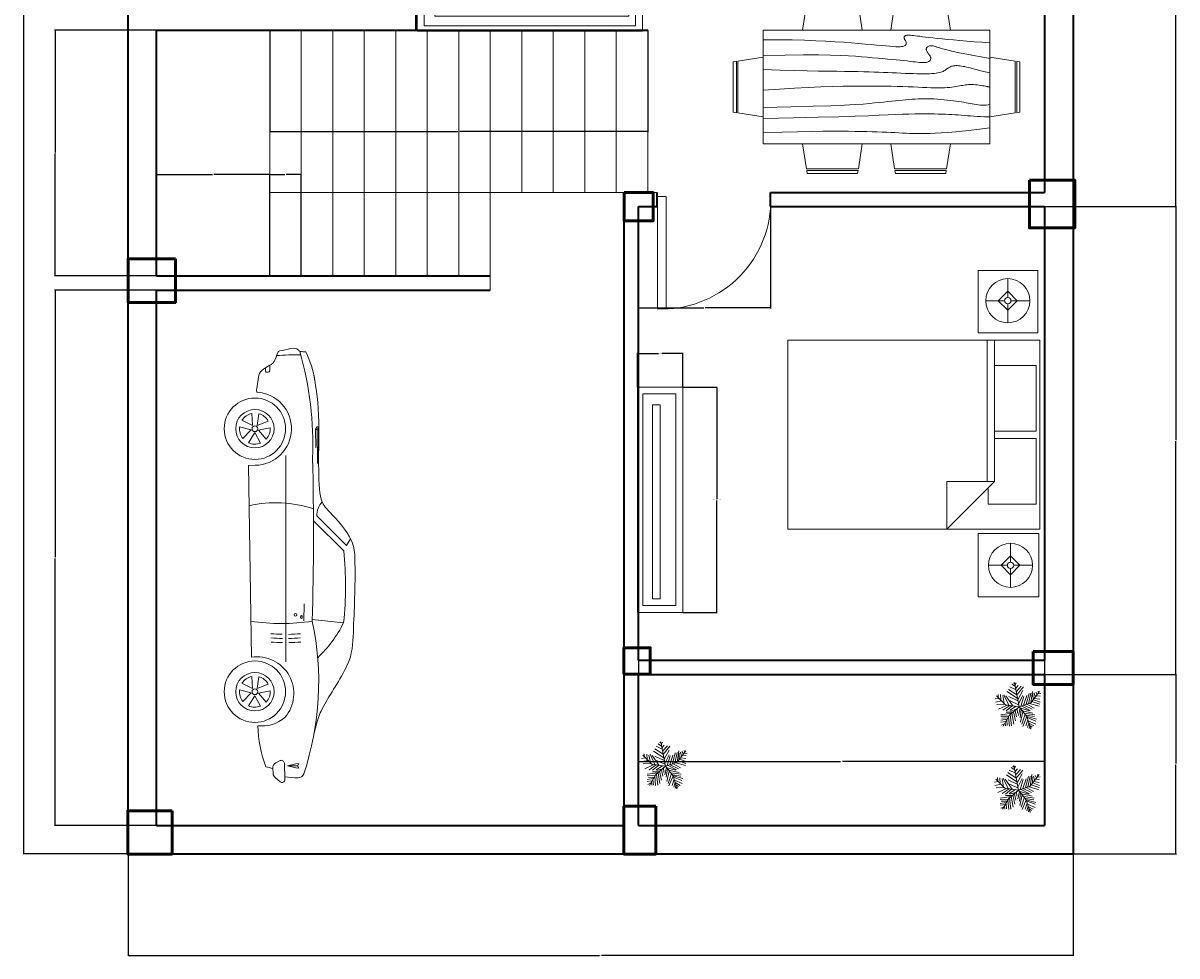
# Model space of a CAD drawing. Units: inches. Extents: x 50 to 2003, y -28 to 675.
# Tile 1 of 10: x 179 to 545, y -15 to 281. Entities that reach past the tile are written whole.
import ezdxf

# ---------------------------------------------------------------- set-up
doc = ezdxf.new("R2010")
doc.units = ezdxf.units.IN
for name, color, linetype, lineweight in [('A-ANNO-DIMS', 2, 'Continuous', 18), ('A-COLS', 1, 'Continuous', 50), ('A-DOOR', 4, 'Continuous', 18), ('A-FLOR-STRS', 4, 'Continuous', 18), ('A-FURN', 8, 'Continuous', 18), ('A-FURN-LITE', 9, 'Continuous', 13), ('A-SITE-VEHC', 8, 'Continuous', 13), ('A-WALL', 7, 'Continuous', 35), ('L-PLNT', 3, 'Continuous', 13)]:
    doc.layers.add(name, color=color, linetype=linetype, lineweight=lineweight)
doc.styles.get("Standard").update_dxf_attribs({"font": 'arial.ttf'})
doc.dimstyles.get("Standard").update_dxf_attribs({"dimtxt": 0.18, "dimasz": 0.18, "dimexe": 0.18, "dimexo": 0.0625, "dimgap": 0.09, "dimtad": 0, "dimtih": 1, "dimtoh": 1, "dimdec": 4, "dimzin": 0, "dimdsep": 46, "dimtxsty": 'Standard', "dimcen": 0.09, "dimadec": 0, "dimazin": 0, "dimtfac": 1, "dimtdec": 4, "dimtofl": 0, "dimtmove": 0, "dimatfit": 3, "dimfxl": 1, "dimtolj": 1, "dimtzin": 0, "dimarcsym": 0})

# ---------------------------------------------------------------- blocks, each defined once
blk = doc.blocks.new('*U4')
for p, q in [((72.93, 40.23), (85.8, 53.18)), ((75, 38.82), (88.08, 51.97)), ((119.39, 51.91), (117.92, 38.32)), ((50.13, 41.06), (34.31, 40.98)), ((35.3, 40.46), (50.13, 40.62)), ((43.26, 39.85), (35.15, 39.78)), ((111.09, 34.73), (118.48, 34.64)), ((46.65, 26.83), (136.29, 26.77)), ((180.37, 26.17), (187.51, 26.41)), ((179.3, 24.35), (180.25, 22.49)), ((182.62, 21.14), (184.91, 21.28)), ((186.68, 22.17), (188.51, 24.37)), ((7.45, 19.78), (9.74, 19.8)), ((9.76, 17.93), (8.53, 17.92)), ((10.37, 19.19), (10.38, 18.56)), ((50.87, 13.52), (50.91, 10.52))]:
    blk.add_line(p, q)
for points in [[(35.31, 39.93), (35.3, 40.27, 0.269532), (35.14, 40.54), (34.38, 40.96, 0.575383), (34.15, 40.83), (34.15, 40.49, 0.269532), (34.32, 40.22), (35.08, 39.79, 0.575383)], [(28.49, 15.1), (33.61, 14.4), (31.65, 19.18, 0.199906)], [(34.64, 20.05), (35.56, 14.97), (39.5, 18.31, 0.199906)], [(41.25, 15.74), (36.7, 13.3), (41.09, 10.58, 0.199906)], [(142.85, 15.1), (147.96, 14.4), (146.01, 19.18, 0.199906)], [(148.99, 20.05), (149.91, 14.97), (153.85, 18.31, 0.199906)], [(155.6, 15.74), (151.06, 13.3), (155.45, 10.58, 0.199906)], [(31.31, 7.72), (33.55, 12.37), (28.4, 11.99, 0.199906)], [(39.19, 8.12), (35.46, 11.69), (34.23, 6.67, 0.199906)], [(145.66, 7.72), (147.9, 12.37), (142.75, 11.99, 0.199906)], [(153.54, 8.12), (149.81, 11.69), (148.59, 6.67, 0.199906)]]:
    blk.add_lwpolyline(points, format="xyb", close=True)
for points in [[(181.58, 27.46), (181.53, 31.95), (180.48, 32.43)], [(181.58, 27.46), (181.53, 31.95), (182.57, 32.45)], [(50.91, 10.52), (134.38, 11.83)]]:
    blk.add_lwpolyline(points)
for centre, radius in [((115.89, 31.01), 0.619), ((34.98, 13.35), 13.35), ((149.33, 13.35), 13.35), ((34.98, 13.35), 8.35), ((149.33, 13.35), 8.35), ((34.98, 13.35), 1.25), ((149.33, 13.35), 1.25)]:
    blk.add_circle(centre, radius)
for centre, radius, start, end in [((114.6, 105.09), 59.37, 237.6103, 240.9785), ((103.45, -95), 147.78, 83.8163, 95.9705), ((95.51, 3.91), 53.61, 43.2748, 63.5665), ((73.29, 50.49), 10.26, 230.424, 268.0085), ((145.17, -84.88), 125.99, 71.5283, 102.1242), ((42.18, -111.35), 149.91, 87.8393, 105.8096), ((20.53, -3.15), 43.06, 98.5304, 116.112), ((80.1, -1364.13), 1402.96, 88.42296, 91.3179), ((118.31, 22.51), 51.16, 161.4307, 193.2363), ((25.66, 24.94), 94.01, 351.8279, 8.1674), ((79.16, 30.11), 76.3, 177.5773, 185.5205), ((45.64, 26.83), 78.76, 0.852, 4.6556), ((47.43, 26.85), 78.76, 0.852, 4.6556), ((49.23, 26.87), 78.76, 0.852, 4.6556), ((150.1, 14.36), 15.92, 49.2263, 189.1528), ((216.26, 37.76), 36.17, 188.4683, 196.5315), ((146.68, 36.98), 36.17, 344.7432, 352.8063), ((184.3, 32.25), 2.49, 357.932, 71.5283), ((116.55, 34.7), 70.29, 353.1942, 357.932), ((34.98, 13.35), 15.9, 0.6373, 176.3412), ((45.64, 26.83), 78.76, 355.2644, 358.8633), ((47.43, 26.85), 78.76, 355.2644, 358.8633), ((49.23, 26.87), 78.76, 355.2644, 358.8633), ((149.4, 16.55), 14.84, 352.7285, 41.6613), ((180.41, 24.92), 1.25, 91.939, 207.109), ((187.55, 25.16), 1.25, 320.1683, 91.939), ((182.47, 23.63), 2.49, 207.109, 273.4677), ((114.25, 37.03), 70.29, 344.3985, 346.9385), ((184.76, 23.76), 2.49, 273.4677, 320.1683), ((9.75, 19.18), 0.623, 0.6373, 90.6373), ((9.76, 18.55), 0.623, 270.6373, 0.6373), ((162.47, 70.82), 56.18, 271.6865, 290.2774)]:
    blk.add_arc(centre, radius, start, end)
blk.add_ellipse((116.89, 33.59), major_axis=(-0.63, -0.007), ratio=0.610043)
for points, knots in [([(11.39, 38.92), (18.06, 40.19), (30.91, 42.01), (64.77, 40.11), (70.25, 44.91), (82.35, 56.38), (99.18, 57.3), (116.06, 56.35), (133.04, 55.87), (145.24, 49.87), (153.62, 43.8), (161.17, 40.68), (164.92, 39.73), (167.29, 39.15)], [18.629823, 18.629823, 18.629823, 18.629823, 19.527405, 20.700571, 21.107983, 21.608568, 21.92336, 23.151359, 23.716171, 23.908743, 24.77794, 24.943072, 25.187755, 25.187755, 25.187755, 25.187755]), ([(19.11, 14.36), (18.99, 14.21), (18.5, 13.81), (15.35, 15), (9.19, 13.94), (7.26, 22.22), (3.01, 22.66), (1.32, 23.61), (0.64, 26.92), (-0.96, 31.49), (1.54, 32.64), (1.5, 34.06), (1.49, 34.8), (1.49, 35.06), (1.52, 35.3), (1.58, 35.51)], [16.815853, 16.815853, 16.815853, 16.815853, 16.838212, 16.885395, 17.18439, 17.479846, 17.654423, 17.670693, 17.696923, 18.016358, 18.052739, 18.140805, 18.140805, 18.140805, 18.172382, 18.172382, 18.172382, 18.172382])]:
    blk.add_open_spline(points, degree=3, knots=knots)
blk = doc.blocks.new('*U2')
for p, q in [((-10.186, 53.64), (-13.084, 55.962)), ((0, 0), (-10.5, 57)), ((-9.099, 51.782), (-6.563, 55.962)), ((-48.585, 21.131), (-49.309, 29.026)), ((-43.513, 28.561), (-42.427, 15.558)), ((-35.544, 28.097), (-24.314, 3.947)), ((-3.665, 19.273), (-27.574, 35.527)), ((-5.114, 28.097), (-24.676, 40.636)), ((-7.288, 39.707), (-21.778, 46.673)), ((-8.737, 47.138), (-17.069, 52.711)), ((-7.65, 43.423), (-2.578, 49.46)), ((-5.839, 35.992), (4.667, 48.067)), ((-5.114, 27.632), (10.463, 46.673)), ((-2.941, 16.486), (8.652, 37.85)), ((16.259, 5.805), (23.142, 31.348)), ((22.055, 7.198), (27.489, 32.277)), ((27, 9), (48, 36)), ((27.127, 9.056), (31.112, 35.992)), ((31.836, 30.883), (32.561, 16.486)), ((35.096, 32.741), (37.27, 22.524)), ((38.719, 34.134), (41.979, 28.561)), ((43.791, 29.954), (51.036, 30.883)), ((44.153, 36.456), (45.239, 32.741)), ((-47.498, 19.737), (-55.83, 18.344)), ((-40.615, 13.7), (-55.105, 10.913)), ((-31.5, 4.5), (-52.5, 25.5)), ((-33.37, 6.269), (-52.207, 5.34)), ((-28.299, 3.483), (-47.86, -5.805)), ((-38.442, 26.239), (-34.819, 7.663)), ((-21.416, 3.018), (-38.079, -8.128)), ((0, 0), (-31.5, 4.5)), ((-14.533, 2.09), (-30.834, 25.31)), ((-15.982, 2.09), (-30.11, -9.521)), ((-24.314, 23.917), (-2.941, 13.7)), ((0, 0), (-22.5, -19.5)), ((-6.563, 1.161), (-21.416, -8.128)), ((-20.691, 13.7), (-1.129, 4.876)), ((-1.129, 6.734), (9.014, 26.704)), ((0, 0), (27, 9)), ((0, 0), (18, -22.5)), ((3.942, 1.625), (11.187, 24.381)), ((6.478, 1.625), (26.04, -8.592)), ((10.101, 3.483), (17.708, 26.239)), ((11.187, 3.483), (30.749, -5.805)), ((18.07, 5.805), (35.096, -3.483)), ((24.229, 7.663), (46.688, 1.625)), ((29.662, 12.307), (48.137, 6.269)), ((33.285, 16.486), (48.862, 10.913)), ((36.183, 19.737), (48.137, 17.88)), ((40.53, 25.775), (48.862, 24.846)), ((-17.431, -15.094), (-42.789, -18.809)), ((-24.314, -21.596), (-42.427, -22.06)), ((-26.849, -26.24), (-40.253, -25.775)), ((-22.5, -19.5), (-37.5, -45)), ((-15.257, -12.772), (-30.11, -12.772)), ((-25.038, -23.918), (-22.865, -45.281)), ((-20.691, -18.345), (-17.793, -44.352)), ((-6.563, -5.805), (-19.967, -9.985)), ((-17.069, -15.094), (-12.721, -40.172)), ((-13.446, -11.378), (-8.737, -32.741)), ((-9.461, -8.592), (-6.201, -23.453)), ((-4.752, -3.483), (-3.665, -14.629)), ((2.493, -3.019), (-1.491, -20.202)), ((1.769, -2.555), (24.229, -9.521)), ((5.029, -6.27), (2.131, -25.775)), ((9.014, -11.378), (3.58, -35.992)), ((14.085, -16.951), (6.478, -40.172)), ((7.565, -9.056), (32.198, -14.629)), ((18.07, -22.524), (8.289, -45.745)), ((12.274, -15.094), (36.907, -18.809)), ((16.259, -19.738), (36.183, -22.989)), ((18, -22.5), (27, -52.5)), ((18.433, -22.524), (40.53, -29.026)), ((19.157, -25.311), (38.719, -33.206)), ((-28.299, -29.026), (-42.789, -31.348)), ((-30.834, -34.135), (-42.427, -35.528)), ((-34.457, -39.708), (-40.978, -42.494)), ((-32.646, -36.921), (-31.921, -44.352)), ((-29.023, -30.884), (-27.936, -43.887)), ((20.244, -30.419), (15.897, -44.816)), ((22.78, -37.85), (19.519, -48.532)), ((21.331, -32.741), (39.081, -40.636)), ((22.78, -38.314), (34.372, -44.816)), ((24.591, -45.745), (23.142, -50.854)), ((24.591, -43.423), (30.749, -47.603)), ((26.764, -49.925), (28.213, -50.854))]:
    blk.add_line(p, q)
blk = doc.blocks.new('Bed - Queen')
for p, q in [((0, -80.00003), (0, 0)), ((0, 0), (59.99999, 0)), ((59.99999, 0), (59.99999, -80.00003)), ((7.99999, -1.2), (28.79998, -1.2)), ((7.99999, -14.4), (7.99999, -1.2)), ((28.79998, -1.2), (28.79998, -14.4)), ((31.19999, -1.2), (51.99999, -1.2)), ((31.19999, -14.4), (31.19999, -1.2)), ((51.99999, -1.2), (51.99999, -16.4)), ((0, -14.4), (44.8, -14.4)), ((59.99999, -29.6), (44.8, -14.4)), ((44.8, -14.4), (44.8, -29.6)), ((44.8, -16.8), (0, -16.8)), ((51.99999, -16.4), (46.79936, -16.4)), ((44.8, -29.6), (59.99999, -29.6)), ((59.99999, -80.00003), (0, -80.00003))]:
    blk.add_line(p, q)
blk = doc.blocks.new('Lamp - Table')
for p, q in [((0, 7), (0, 1)), ((-1, 0), (-7, 0)), ((0, 3), (-3, 0)), ((-3, 0), (0, -3)), ((3, 0), (0, 3)), ((0, -3), (3, 0)), ((1, 0), (7, 0)), ((0, -1), (0, -7))]:
    blk.add_line(p, q)
for radius in [7, 1]:
    blk.add_circle((0, 0), radius)
blk = doc.blocks.new('Dining Set - 36 x 72 in.')
for p, q in [((-22.2343, 26.00059), (-23.4847, 17.99762)), ((-22.2304, 26), (-5.7608, 26)), ((-22, 27.5), (-22.1562, 26.50042)), ((-5.8416, 26.5), (-22.1534, 26.5)), ((-22, 27.5), (-6, 27.5)), ((-5.8437, 26.49966), (-6, 27.5)), ((-4.5152, 17.99762), (-5.7655, 25.99926)), ((5.7657, 26.00059), (4.5153, 17.99762)), ((5.7696, 26), (22.2392, 26)), ((6, 27.5), (5.8438, 26.50042)), ((22.1584, 26.5), (5.8466, 26.5)), ((6, 27.5), (22, 27.5)), ((22.1563, 26.49966), (22, 27.5)), ((23.4848, 17.99762), (22.2345, 25.99926)), ((36, 18), (-36, 18)), ((-36, 18), (-36, -18)), ((36, -18), (36, 18)), ((-45.5, 8), (-44.5004, 8.15617)), ((-45.5, 8), (-45.5, -8)), ((-44.5, -8.15843), (-44.5, 8.15338)), ((-44.0006, 8.23428), (-35.9976, 9.48474)), ((-44, 8.23041), (-44, -8.23915)), ((44.0006, 8.23428), (35.9976, 9.48474)), ((44, 8.23041), (44, -8.23915)), ((44.5, -8.15843), (44.5, 8.15338)), ((45.5, 8), (44.5005, 8.15617)), ((45.5, 8), (45.5, -8)), ((-44.4997, -8.15631), (-45.5, -8)), ((-35.9976, -9.48476), (-43.9993, -8.2345)), ((35.9976, -9.48476), (43.9993, -8.2345)), ((44.4997, -8.15631), (45.5, -8)), ((-36, -18), (36, -18)), ((-22.2343, -26.0006), (-23.4847, -17.99762)), ((-4.5152, -17.99762), (-5.7655, -25.99928)), ((5.7657, -26.0006), (4.5153, -17.99762)), ((23.4848, -17.99762), (22.2345, -25.99928)), ((-22.2304, -26), (-5.7608, -26)), ((-22, -27.5), (-22.1562, -26.50044)), ((-5.8416, -26.5), (-22.1534, -26.5)), ((-22, -27.5), (-6, -27.5)), ((-5.8437, -26.49967), (-6, -27.5)), ((5.7696, -26), (22.2392, -26)), ((6, -27.5), (5.8438, -26.50044)), ((22.1584, -26.5), (5.8466, -26.5)), ((6, -27.5), (22, -27.5)), ((22.1563, -26.49967), (22, -27.5))]:
    blk.add_line(p, q)
for points in [[(-36, 15), (-31.1772, 14.97754), (-26.8079, 14.91406), (-22.8538, 14.81543), (-19.276, 14.6875), (-16.0362, 14.53613), (-13.0957, 14.36718), (-10.4159, 14.18652), (-7.9583, 14), (-5.6904, 13.81315), (-3.6035, 13.63021), (-1.6954, 13.45508), (0.0365, 13.29166), (1.5945, 13.14388), (2.9811, 13.01562), (4.1988, 12.9108), (5.25, 12.83333), (6.1393, 12.78613), (6.8802, 12.76823), (7.4883, 12.77767), (7.9792, 12.8125), (8.3685, 12.87077), (8.6719, 12.95052), (8.9049, 13.0498), (9.0833, 13.16666), (9.2205, 13.29899), (9.3216, 13.44401), (9.3895, 13.59879), (9.4271, 13.76041), (9.4373, 13.92594), (9.4232, 14.09245), (9.3875, 14.257), (9.3333, 14.41666), (9.2638, 14.56917), (9.1836, 14.71484), (9.0975, 14.85465), (9.0104, 14.98958), (8.9272, 15.1206), (8.8529, 15.2487), (8.7922, 15.37483), (8.75, 15.5), (8.7305, 15.62467), (8.7344, 15.74739), (8.7617, 15.86621), (8.8125, 15.97916), (8.8867, 16.08431), (8.9844, 16.17968), (9.1055, 16.26334), (9.25, 16.33333), (9.4189, 16.38802), (9.6172, 16.42708), (9.8506, 16.45052), (10.125, 16.45833), (10.4463, 16.45052), (10.8203, 16.42708), (11.2529, 16.38802), (11.75, 16.33333), (12.3184, 16.26318), (12.9694, 16.17838), (13.7151, 16.07991), (14.5677, 15.96875), (15.5395, 15.84586), (16.6426, 15.71224), (17.8893, 15.56884), (19.2917, 15.41666), (20.859, 15.25667), (22.5879, 15.08984), (24.4721, 14.91715), (26.5052, 14.73958), (28.6809, 14.5581), (30.9929, 14.3737), (33.4347, 14.18733), (36, 14)], [(-36, 10), (-28.9766, 10.14274), (-23.1725, 10.20442), (-18.4241, 10.19775), (-14.5677, 10.13541), (-11.4399, 10.03011), (-8.877, 9.89453), (-6.7154, 9.74137), (-4.7917, 9.58333), (-2.9698, 9.43082), (-1.2246, 9.28515), (0.4415, 9.14534), (2.026, 9.01041), (3.5266, 8.87939), (4.9408, 8.7513), (6.266, 8.62516), (7.5, 8.5), (8.6411, 8.37549), (9.6914, 8.2539), (10.6538, 8.13818), (11.5312, 8.03125), (12.3267, 7.93603), (13.043, 7.85547), (13.6831, 7.79248), (14.25, 7.75), (14.7471, 7.7303), (15.1797, 7.73307), (15.5537, 7.75732), (15.875, 7.80208), (16.1494, 7.86637), (16.3828, 7.94922), (16.5811, 8.04964), (16.75, 8.16666), (16.8944, 8.29915), (17.0143, 8.44531), (17.1089, 8.60319), (17.1771, 8.77083), (17.218, 8.94629), (17.2305, 9.1276), (17.2137, 9.31282), (17.1667, 9.5), (17.0895, 9.6875), (16.987, 9.875), (16.8649, 10.0625), (16.7292, 10.25), (16.5856, 10.4375), (16.4401, 10.625), (16.2985, 10.8125), (16.1667, 11), (16.05, 11.18733), (15.9518, 11.3737), (15.8752, 11.5581), (15.8229, 11.73958), (15.798, 11.91715), (15.8034, 12.08984), (15.842, 12.25667), (15.9167, 12.41666), (16.0295, 12.56836), (16.1784, 12.70833), (16.3605, 12.83268), (16.5729, 12.9375), (16.8127, 13.01888), (17.0768, 13.07291), (17.3625, 13.0957), (17.6667, 13.08333), (17.9894, 13.03312), (18.3418, 12.94726), (18.7382, 12.82918), (19.1927, 12.68229), (19.7195, 12.51001), (20.3327, 12.31575), (21.0465, 12.10294), (21.875, 11.875), (22.8357, 11.63354), (23.959, 11.37304), (25.2786, 11.08618), (26.8282, 10.76562), (28.6414, 10.40405), (30.752, 9.99414), (33.1936, 9.52856), (36, 9)], [(-36, 5.5), (-30.7157, 5.3348), (-26.069, 5.20963), (-21.9946, 5.11767), (-18.4271, 5.05208), (-15.3009, 5.00602), (-12.5508, 4.97265), (-10.1112, 4.94515), (-7.9167, 4.91666), (-5.909, 4.88167), (-4.0586, 4.83984), (-2.3429, 4.79215), (-0.7396, 4.73958), (0.7739, 4.6831), (2.22, 4.6237), (3.6213, 4.56233), (5, 4.5), (6.373, 4.43782), (7.7344, 4.3776), (9.0723, 4.32129), (10.375, 4.27083), (11.6309, 4.22819), (12.8281, 4.19531), (13.9551, 4.17415), (15, 4.16666), (15.954, 4.17448), (16.819, 4.19791), (17.6001, 4.23698), (18.3021, 4.29166), (18.9299, 4.36198), (19.4883, 4.44791), (19.9823, 4.54948), (20.4167, 4.66666), (20.7969, 4.79899), (21.1302, 4.94401), (21.4245, 5.09879), (21.6875, 5.26041), (21.9271, 5.42594), (22.1511, 5.59245), (22.3672, 5.757), (22.5834, 5.91666), (22.8065, 6.06868), (23.0404, 6.21093), (23.2879, 6.34147), (23.5521, 6.45833), (23.8358, 6.55957), (24.142, 6.64323), (24.4735, 6.70735), (24.8334, 6.75), (25.2235, 6.76969), (25.642, 6.76692), (26.0858, 6.74267), (26.5521, 6.69791), (27.0379, 6.63362), (27.5404, 6.55078), (28.0565, 6.45036), (28.5834, 6.33333), (29.1242, 6.19987), (29.7071, 6.04687), (30.3661, 5.87044), (31.1354, 5.66666), (32.0493, 5.43164), (33.142, 5.16146), (34.4475, 4.85221), (36, 4.5)], [(-36, -1), (-30.7915, -0.6591), (-26.0195, -0.38216), (-21.6519, -0.16284), (-17.6563, 0.00521), (-14.0005, 0.12833), (-10.6523, 0.21289), (-7.5796, 0.26522), (-4.75, 0.29166), (-2.134, 0.29793), (0.2878, 0.28711), (2.5317, 0.26163), (4.6146, 0.22396), (6.5529, 0.17651), (8.3633, 0.12174), (10.0623, 0.06209), (11.6667, 0), (13.1899, -0.06201), (14.6341, -0.1211), (15.9982, -0.17432), (17.2813, -0.21875), (18.4823, -0.25147), (19.6003, -0.26953), (20.6343, -0.27002), (21.5834, -0.25), (22.4481, -0.20768), (23.2357, -0.14584), (23.9549, -0.06836), (24.6146, 0.02083), (25.2235, 0.11784), (25.7904, 0.21875), (26.3241, 0.31966), (26.8334, 0.41666), (27.3265, 0.50618), (27.8099, 0.58593), (28.2894, 0.65397), (28.7709, 0.70833), (29.2601, 0.74707), (29.763, 0.76823), (30.2855, 0.76985), (30.8334, 0.75), (31.4088, 0.70784), (31.9994, 0.64713), (32.589, 0.57275), (33.1615, 0.48958), (33.7008, 0.4025), (34.1908, 0.3164), (34.6153, 0.23616), (34.9584, 0.16666), (35.2099, 0.11165), (35.3848, 0.07031), (35.504, 0.04069), (35.5886, 0.02083), (35.6594, 0.00879), (35.7377, 0.0026), (35.8442, 0.00032), (36, 0)], [(-36, -6.5), (-27.1843, -6.31267), (-20.084, -6.1263), (-14.469, -5.9419), (-10.1094, -5.76042), (-6.7752, -5.58285), (-4.2363, -5.41016), (-2.2629, -5.24333), (-0.625, -5.08334), (0.8708, -4.93099), (2.2715, -4.78646), (3.5872, -4.64974), (4.8281, -4.52084), (6.0046, -4.39974), (7.127, -4.28646), (8.2053, -4.18099), (9.25, -4.08334), (10.2705, -3.99382), (11.2734, -3.91407), (12.2647, -3.84603), (13.25, -3.79167), (14.2354, -3.75293), (15.2266, -3.73177), (16.2295, -3.73015), (17.25, -3.75), (18.2912, -3.79248), (19.3451, -3.85547), (20.4009, -3.93604), (21.4479, -4.03125), (22.4754, -4.13819), (23.4727, -4.25391), (24.4289, -4.37549), (25.3334, -4.5), (26.1785, -4.62492), (26.9694, -4.74935), (27.7145, -4.87281), (28.4219, -4.99479), (29.1, -5.11483), (29.7572, -5.23242), (30.4016, -5.34709), (31.0417, -5.45834), (31.6837, -5.56437), (32.3262, -5.65821), (32.9658, -5.73153), (33.599, -5.77604), (34.2224, -5.78345), (34.8327, -5.74545), (35.4264, -5.65373), (36, -5.5)], [(-36, -10), (-26.4022, -9.81299), (-18.4675, -9.62891), (-11.9839, -9.45069), (-6.7396, -9.28125), (-2.5226, -9.12354), (0.8789, -8.98047), (3.6769, -8.85498), (6.0833, -8.75), (8.2767, -8.66765), (10.3021, -8.60677), (12.1712, -8.56543), (13.8958, -8.54167), (15.4876, -8.53353), (16.9583, -8.53907), (18.3197, -8.55632), (19.5834, -8.58334), (20.7616, -8.61841), (21.8685, -8.66081), (22.9188, -8.71004), (23.9271, -8.76563), (24.9081, -8.82707), (25.8763, -8.89388), (26.8465, -8.96558), (27.8334, -9.04167), (28.8474, -9.12118), (29.8828, -9.20117), (30.93, -9.27824), (31.9792, -9.34896), (33.0205, -9.40991), (34.0443, -9.45768), (35.0407, -9.48885), (36, -9.5)], [(-36, -14.5), (-30.0881, -14.33513), (-25.0332, -14.21224), (-20.7312, -14.12647), (-17.0781, -14.07292), (-13.97, -14.04671), (-11.3027, -14.04297), (-8.9724, -14.05681), (-6.875, -14.08334), (-4.9224, -14.11833), (-3.0905, -14.16016), (-1.3709, -14.20785), (0.2448, -14.26042), (1.7647, -14.3169), (3.1973, -14.3763), (4.5507, -14.43767), (5.8333, -14.5), (7.0554, -14.5621), (8.235, -14.62175), (9.3922, -14.67652), (10.5469, -14.72396), (11.7192, -14.76164), (12.929, -14.78711), (14.1965, -14.79794), (15.5417, -14.79167), (16.9933, -14.76424), (18.6152, -14.70508), (20.4804, -14.60197), (22.6615, -14.44271), (25.2312, -14.21509), (28.2624, -13.9069), (31.8277, -13.50594), (36, -13)]]:
    blk.add_lwpolyline(points)
blk = doc.blocks.new('MEDIA-CONSOLE')
for points in [[(0, 0), (71.49, 0), (71.49, 14.4), (0, 14.4)], [(2.13, 1.7), (69.3, 1.7), (69.3, 12.15), (2.13, 12.15)], [(5.56, 4.74), (67.2, 4.74), (67.2, 7.16), (5.56, 7.16)]]:
    blk.add_lwpolyline(points, close=True)
blk = doc.blocks.new('DOOR-LEAF-36')
blk.add_lwpolyline([(35.71, 2.81), (35.71, 0), (0, 0), (0, 2.81)], close=True)
blk = doc.blocks.new('NIGHTSTAND-COMPACT')
blk.add_lwpolyline([(0, 19.73), (0, 0), (18.92, 0), (18.92, 19.73)], close=True)
blk = doc.blocks.new('NIGHTSTAND-STANDARD')
blk.add_lwpolyline([(0, 0), (0, 20.13), (19.19, 20.13), (19.19, 0)], close=True)
blk = doc.blocks.new('*D33')
at = {"layer": 'A-ANNO-DIMS', "color": 0, "lineweight": -2, "transparency": 16777216}
for p, q in [((388.19, 165.48), (399.03, 165.48)), ((398.85, 165.3), (398.85, 129.92)), ((398.85, 94.17), (398.85, 129.55)), ((388.19, 93.99), (399.03, 93.99))]:
    blk.add_line(p, q, dxfattribs=at)
at = {"layer": 'A-ANNO-DIMS', "color": 0, "transparency": 16777216}
for points in [[(398.82, 165.3), (398.88, 165.3), (398.85, 165.48)], [(398.82, 94.17), (398.88, 94.17), (398.85, 93.99)]]:
    blk.add_solid(points, dxfattribs=at)
at = {"layer": 'Defpoints', "color": 0, "transparency": 16777216}
for p in [(388.13, 165.48), (388.13, 93.99), (398.85, 93.99)]:
    blk.add_point(p, dxfattribs=at)
at = {"layer": 'A-ANNO-DIMS', "color": 0, "transparency": 16777216, "insert": (398.85, 129.74), "char_height": 0.18, "attachment_point": 5}
blk.add_mtext('\\A1;MEDIA CONSOLE 71 TYP.', dxfattribs=at)
blk = doc.blocks.new('*D34')
at = {"layer": 'A-ANNO-DIMS', "color": 0, "lineweight": -2, "transparency": 16777216}
for p, q in [((373.72, 165.54), (373.72, 176.38)), ((373.9, 176.2), (380.4, 176.2)), ((387.95, 176.2), (381.44, 176.2)), ((388.13, 165.54), (388.13, 176.38))]:
    blk.add_line(p, q, dxfattribs=at)
at = {"layer": 'A-ANNO-DIMS', "color": 0, "transparency": 16777216}
for points in [[(373.9, 176.23), (373.9, 176.17), (373.72, 176.2)], [(387.95, 176.23), (387.95, 176.17), (388.13, 176.2)]]:
    blk.add_solid(points, dxfattribs=at)
at = {"layer": 'Defpoints', "color": 0, "transparency": 16777216}
for p in [(388.13, 176.2), (373.72, 165.48), (388.13, 165.48)]:
    blk.add_point(p, dxfattribs=at)
at = {"layer": 'A-ANNO-DIMS', "color": 0, "transparency": 16777216, "insert": (380.92, 176.2), "char_height": 0.18, "attachment_point": 5}
blk.add_mtext('\\A1;14 TYP.', dxfattribs=at)
blk = doc.blocks.new('*D51')
at = {"layer": 'A-ANNO-DIMS', "color": 0, "lineweight": -2, "transparency": 16777216}
for p, q in [((211.97, 17.26), (211.97, -15.05)), ((511.97, 17.26), (511.97, -15.05)), ((212.15, -14.87), (361.68, -14.87)), ((511.79, -14.87), (362.26, -14.87))]:
    blk.add_line(p, q, dxfattribs=at)
at = {"layer": 'A-ANNO-DIMS', "color": 0, "transparency": 16777216}
for points in [[(212.15, -14.84), (212.15, -14.9), (211.97, -14.87)], [(511.79, -14.84), (511.79, -14.9), (511.97, -14.87)]]:
    blk.add_solid(points, dxfattribs=at)
at = {"layer": 'Defpoints', "color": 0, "transparency": 16777216}
for p in [(211.97, 17.32), (511.97, 17.32), (511.97, -14.87)]:
    blk.add_point(p, dxfattribs=at)
at = {"layer": 'A-ANNO-DIMS', "color": 0, "transparency": 16777216, "insert": (361.97, -14.87), "char_height": 0.18, "attachment_point": 5}
blk.add_mtext('\\A1;300', dxfattribs=at)
blk = doc.blocks.new('*D52')
at = {"layer": 'A-ANNO-DIMS', "color": 0, "lineweight": -2, "transparency": 16777216}
for p, q in [((211.91, 642.32), (178.66, 642.32)), ((178.84, 642.14), (178.84, 330.01)), ((178.84, 17.5), (178.84, 329.64)), ((211.91, 17.32), (178.66, 17.32))]:
    blk.add_line(p, q, dxfattribs=at)
at = {"layer": 'A-ANNO-DIMS', "color": 0, "transparency": 16777216}
for points in [[(178.81, 642.14), (178.87, 642.14), (178.84, 642.32)], [(178.81, 17.5), (178.87, 17.5), (178.84, 17.32)]]:
    blk.add_solid(points, dxfattribs=at)
at = {"layer": 'Defpoints', "color": 0, "transparency": 16777216}
for p in [(178.84, 642.32), (211.97, 642.32), (211.97, 17.32)]:
    blk.add_point(p, dxfattribs=at)
at = {"layer": 'A-ANNO-DIMS', "color": 0, "transparency": 16777216, "insert": (178.84, 329.82), "char_height": 0.18, "attachment_point": 5}
blk.add_mtext('\\A1;625', dxfattribs=at)
blk = doc.blocks.new('*D53')
at = {"layer": 'A-ANNO-DIMS', "color": 0, "lineweight": -2, "transparency": 16777216}
for p, q in [((373.97, 78.76), (373.97, 46.49)), ((502.97, 78.76), (502.97, 46.49)), ((374.15, 46.67), (438.19, 46.67)), ((502.79, 46.67), (438.75, 46.67))]:
    blk.add_line(p, q, dxfattribs=at)
at = {"layer": 'A-ANNO-DIMS', "color": 0, "transparency": 16777216}
for points in [[(374.15, 46.7), (374.15, 46.64), (373.97, 46.67)], [(502.79, 46.7), (502.79, 46.64), (502.97, 46.67)]]:
    blk.add_solid(points, dxfattribs=at)
at = {"layer": 'Defpoints', "color": 0, "transparency": 16777216}
for p in [(373.97, 78.82), (502.97, 78.82), (373.97, 46.67)]:
    blk.add_point(p, dxfattribs=at)
at = {"layer": 'A-ANNO-DIMS', "color": 0, "transparency": 16777216, "insert": (438.47, 46.67), "char_height": 0.18, "attachment_point": 5}
blk.add_mtext('\\A1;129', dxfattribs=at)
blk = doc.blocks.new('*D59')
at = {"layer": 'A-ANNO-DIMS', "color": 0, "lineweight": -2, "transparency": 16777216}
for p, q in [((503.03, 74.32), (544.84, 74.32)), ((544.66, 74.14), (544.66, 46)), ((544.66, 17.5), (544.66, 45.64)), ((512.03, 17.32), (544.84, 17.32))]:
    blk.add_line(p, q, dxfattribs=at)
at = {"layer": 'A-ANNO-DIMS', "color": 0, "transparency": 16777216}
for points in [[(544.63, 74.14), (544.69, 74.14), (544.66, 74.32)], [(544.63, 17.5), (544.69, 17.5), (544.66, 17.32)]]:
    blk.add_solid(points, dxfattribs=at)
at = {"layer": 'Defpoints', "color": 0, "transparency": 16777216}
for p in [(502.97, 74.32), (544.66, 74.32), (511.97, 17.32)]:
    blk.add_point(p, dxfattribs=at)
at = {"layer": 'A-ANNO-DIMS', "color": 0, "transparency": 16777216, "insert": (544.66, 45.82), "char_height": 0.18, "attachment_point": 5}
blk.add_mtext('\\A1;57', dxfattribs=at)
blk = doc.blocks.new('*D60')
at = {"layer": 'A-ANNO-DIMS', "color": 0, "lineweight": -2, "transparency": 16777216}
for p, q in [((503.03, 222.82), (544.84, 222.82)), ((544.66, 222.64), (544.66, 148.76)), ((544.66, 74.5), (544.66, 148.39)), ((503.03, 74.32), (544.84, 74.32))]:
    blk.add_line(p, q, dxfattribs=at)
at = {"layer": 'A-ANNO-DIMS', "color": 0, "transparency": 16777216}
for points in [[(544.63, 222.64), (544.69, 222.64), (544.66, 222.82)], [(544.63, 74.5), (544.69, 74.5), (544.66, 74.32)]]:
    blk.add_solid(points, dxfattribs=at)
at = {"layer": 'Defpoints', "color": 0, "transparency": 16777216}
for p in [(502.97, 222.82), (544.66, 222.82), (502.97, 74.32)]:
    blk.add_point(p, dxfattribs=at)
at = {"layer": 'A-ANNO-DIMS', "color": 0, "transparency": 16777216, "insert": (544.66, 148.57), "char_height": 0.18, "attachment_point": 5}
blk.add_mtext('\\A1;148.5', dxfattribs=at)
blk = doc.blocks.new('*D61')
at = {"layer": 'A-ANNO-DIMS', "color": 0, "lineweight": -2, "transparency": 16777216}
for p, q in [((503.03, 391.32), (544.84, 391.32)), ((544.66, 391.14), (544.66, 307.26)), ((544.66, 223), (544.66, 306.89)), ((503.03, 222.82), (544.84, 222.82))]:
    blk.add_line(p, q, dxfattribs=at)
at = {"layer": 'A-ANNO-DIMS', "color": 0, "transparency": 16777216}
for points in [[(544.63, 391.14), (544.69, 391.14), (544.66, 391.32)], [(544.63, 223), (544.69, 223), (544.66, 222.82)]]:
    blk.add_solid(points, dxfattribs=at)
at = {"layer": 'Defpoints', "color": 0, "transparency": 16777216}
for p in [(502.97, 391.32), (544.66, 391.32), (502.97, 222.82)]:
    blk.add_point(p, dxfattribs=at)
at = {"layer": 'A-ANNO-DIMS', "color": 0, "transparency": 16777216, "insert": (544.66, 307.07), "char_height": 0.18, "attachment_point": 5}
blk.add_mtext('\\A1;168.5', dxfattribs=at)
blk = doc.blocks.new('*D64')
at = {"layer": 'A-ANNO-DIMS', "color": 0, "lineweight": -2, "transparency": 16777216}
for p, q in [((220.91, 196.32), (188.64, 196.32)), ((188.82, 196.14), (188.82, 111.51)), ((188.82, 26.5), (188.82, 111.14)), ((220.91, 26.32), (188.64, 26.32))]:
    blk.add_line(p, q, dxfattribs=at)
at = {"layer": 'A-ANNO-DIMS', "color": 0, "transparency": 16777216}
for points in [[(188.79, 196.14), (188.85, 196.14), (188.82, 196.32)], [(188.79, 26.5), (188.85, 26.5), (188.82, 26.32)]]:
    blk.add_solid(points, dxfattribs=at)
at = {"layer": 'Defpoints', "color": 0, "transparency": 16777216}
for p in [(188.82, 196.32), (220.97, 196.32), (220.97, 26.32)]:
    blk.add_point(p, dxfattribs=at)
at = {"layer": 'A-ANNO-DIMS', "color": 0, "transparency": 16777216, "insert": (188.82, 111.32), "char_height": 0.18, "attachment_point": 5}
blk.add_mtext('\\A1;170', dxfattribs=at)
blk = doc.blocks.new('*D65')
at = {"layer": 'A-ANNO-DIMS', "color": 0, "lineweight": -2, "transparency": 16777216}
for p, q in [((220.91, 278.82), (188.64, 278.82)), ((188.82, 278.64), (188.82, 240.01)), ((188.82, 201), (188.82, 239.64)), ((220.91, 200.82), (188.64, 200.82))]:
    blk.add_line(p, q, dxfattribs=at)
at = {"layer": 'A-ANNO-DIMS', "color": 0, "transparency": 16777216}
for points in [[(188.79, 278.64), (188.85, 278.64), (188.82, 278.82)], [(188.79, 201), (188.85, 201), (188.82, 200.82)]]:
    blk.add_solid(points, dxfattribs=at)
at = {"layer": 'Defpoints', "color": 0, "transparency": 16777216}
for p in [(188.82, 278.82), (220.97, 278.82), (220.97, 200.82)]:
    blk.add_point(p, dxfattribs=at)
at = {"layer": 'A-ANNO-DIMS', "color": 0, "transparency": 16777216, "insert": (188.82, 239.82), "char_height": 0.18, "attachment_point": 5}
blk.add_mtext('\\A1;78', dxfattribs=at)
blk = doc.blocks.new('*D66')
at = {"layer": 'A-ANNO-DIMS', "color": 0, "lineweight": -2, "transparency": 16777216}
for p, q in [((220.97, 200.89), (220.97, 233.15)), ((221.15, 232.97), (238.75, 232.97)), ((256.79, 232.97), (239.19, 232.97)), ((256.97, 200.89), (256.97, 233.15))]:
    blk.add_line(p, q, dxfattribs=at)
at = {"layer": 'A-ANNO-DIMS', "color": 0, "transparency": 16777216}
for points in [[(221.15, 233), (221.15, 232.94), (220.97, 232.97)], [(256.79, 233), (256.79, 232.94), (256.97, 232.97)]]:
    blk.add_solid(points, dxfattribs=at)
at = {"layer": 'Defpoints', "color": 0, "transparency": 16777216}
for p in [(256.97, 232.97), (220.97, 200.82), (256.97, 200.82)]:
    blk.add_point(p, dxfattribs=at)
at = {"layer": 'A-ANNO-DIMS', "color": 0, "transparency": 16777216, "insert": (238.97, 232.97), "char_height": 0.18, "attachment_point": 5}
blk.add_mtext('\\A1;36', dxfattribs=at)
blk = doc.blocks.new('*D67')
at = {"layer": 'A-ANNO-DIMS', "color": 0, "lineweight": -2, "transparency": 16777216}
for p, q in [((256.97, 200.89), (256.97, 233.15)), ((257.15, 232.97), (261.76, 232.97)), ((266.79, 232.97), (262.18, 232.97)), ((266.97, 200.89), (266.97, 233.15))]:
    blk.add_line(p, q, dxfattribs=at)
at = {"layer": 'A-ANNO-DIMS', "color": 0, "transparency": 16777216}
for points in [[(257.15, 233), (257.15, 232.94), (256.97, 232.97)], [(266.79, 233), (266.79, 232.94), (266.97, 232.97)]]:
    blk.add_solid(points, dxfattribs=at)
at = {"layer": 'Defpoints', "color": 0, "transparency": 16777216}
for p in [(266.97, 232.97), (256.97, 200.82), (266.97, 200.82)]:
    blk.add_point(p, dxfattribs=at)
at = {"layer": 'A-ANNO-DIMS', "color": 0, "transparency": 16777216, "insert": (261.97, 232.97), "char_height": 0.18, "attachment_point": 5}
blk.add_mtext('\\A1;10', dxfattribs=at)
blk = doc.blocks.new('*D68')
at = {"layer": 'A-ANNO-DIMS', "color": 0, "lineweight": -2, "transparency": 16777216}
for p, q in [((256.97, 278.76), (256.97, 246.49)), ((376.97, 278.76), (376.97, 246.49)), ((257.15, 246.67), (316.69, 246.67)), ((376.79, 246.67), (317.25, 246.67))]:
    blk.add_line(p, q, dxfattribs=at)
at = {"layer": 'A-ANNO-DIMS', "color": 0, "transparency": 16777216}
for points in [[(257.15, 246.7), (257.15, 246.64), (256.97, 246.67)], [(376.79, 246.7), (376.79, 246.64), (376.97, 246.67)]]:
    blk.add_solid(points, dxfattribs=at)
at = {"layer": 'Defpoints', "color": 0, "transparency": 16777216}
for p in [(256.97, 278.82), (376.97, 278.82), (256.97, 246.67)]:
    blk.add_point(p, dxfattribs=at)
at = {"layer": 'A-ANNO-DIMS', "color": 0, "transparency": 16777216, "insert": (316.97, 246.67), "char_height": 0.18, "attachment_point": 5}
blk.add_mtext('\\A1;120', dxfattribs=at)
blk = doc.blocks.new('*D71')
at = {"layer": 'A-ANNO-DIMS', "color": 0, "lineweight": -2, "transparency": 16777216}
for p, q in [((373.97, 222.76), (373.97, 190.49)), ((415.97, 222.76), (415.97, 190.49)), ((374.15, 190.67), (394.75, 190.67)), ((415.79, 190.67), (395.19, 190.67))]:
    blk.add_line(p, q, dxfattribs=at)
at = {"layer": 'A-ANNO-DIMS', "color": 0, "transparency": 16777216}
for points in [[(374.15, 190.7), (374.15, 190.64), (373.97, 190.67)], [(415.79, 190.7), (415.79, 190.64), (415.97, 190.67)]]:
    blk.add_solid(points, dxfattribs=at)
at = {"layer": 'Defpoints', "color": 0, "transparency": 16777216}
for p in [(373.97, 222.82), (415.97, 222.82), (373.97, 190.67)]:
    blk.add_point(p, dxfattribs=at)
at = {"layer": 'A-ANNO-DIMS', "color": 0, "transparency": 16777216, "insert": (394.97, 190.67), "char_height": 0.18, "attachment_point": 5}
blk.add_mtext('\\A1;42', dxfattribs=at)

msp = doc.modelspace()

# ---------------------------------------------------------------- linework, layer by layer
at = {"layer": 'A-COLS'}
for points in [[(498.1161, 231.2551), (512.5051, 231.2551), (512.5051, 216.0406), (498.1161, 216.0406)], [(369.4344, 227.2729), (378.6859, 227.2729), (378.6859, 218.3074), (369.4344, 218.3074)], [(227.0033, 206.2582), (211.987, 206.2582), (211.987, 192.4057), (227.0033, 192.4057)], [(369.3824, 74.3697), (377.7786, 74.3697), (377.7786, 82.7607), (369.3824, 82.7607)], [(499.3477, 81.5888), (511.9735, 81.5888), (511.9735, 71.1213), (499.3477, 71.1213)], [(225.9277, 30.9969), (211.8707, 30.9969), (211.8707, 17.2755), (225.9277, 17.2755)], [(379.497, 32.4542), (369.4042, 32.4542), (369.4042, 17.2919), (379.497, 17.2919)]]:
    msp.add_lwpolyline(points, close=True, dxfattribs=at)
at = {"layer": 'A-DOOR'}
msp.add_arc((381.4549, 224.8983), 34.5853, 267.473261, 358.439455, dxfattribs=at)
at = {"layer": 'A-FLOR-STRS'}
for p, q in [((256.9711, 200.8232), (256.9711, 278.8232)), ((266.9711, 200.8232), (266.9711, 278.8232)), ((276.9711, 200.8232), (276.9711, 278.8232)), ((286.9711, 200.8232), (286.9711, 278.8232)), ((296.9711, 200.8232), (296.9711, 278.8232)), ((306.9711, 200.8232), (306.9711, 278.8232)), ((316.9711, 200.8232), (316.9711, 278.8232)), ((326.9711, 196.3232), (326.9711, 278.8232)), ((336.9711, 227.3232), (336.9711, 278.8232)), ((346.9711, 227.3232), (346.9711, 278.8232)), ((356.9711, 227.3232), (356.9711, 278.8232)), ((366.9711, 227.3232), (366.9711, 278.8232)), ((376.9711, 227.3232), (376.9711, 278.8232)), ((256.9711, 227.3232), (379.9711, 227.3232))]:
    msp.add_line(p, q, dxfattribs=at)
at = {"layer": 'A-WALL'}
for p, q in [((211.9711, 17.3232), (211.9711, 642.3232)), ((511.9711, 642.3232), (511.9711, 17.3232)), ((502.9711, 391.3232), (502.9711, 227.3232)), ((303.4711, 278.8232), (303.4711, 331.3232)), ((220.9711, 278.8232), (376.9711, 278.8232)), ((220.9711, 200.8232), (220.9711, 278.8232)), ((369.4711, 26.3232), (369.4711, 227.3232)), ((379.9711, 222.8232), (379.9711, 227.3232)), ((415.9711, 222.8232), (415.9711, 227.3232)), ((415.9711, 227.3232), (502.9711, 227.3232)), ((373.9711, 222.8232), (379.9711, 222.8232)), ((373.9711, 78.8232), (373.9711, 222.8232)), ((415.9711, 222.8232), (502.9711, 222.8232)), ((502.9711, 222.8232), (502.9711, 78.8232)), ((220.9711, 200.8232), (326.9711, 200.8232)), ((220.9711, 26.3232), (220.9711, 196.3232)), ((220.9711, 196.3232), (326.9711, 196.3232)), ((373.9711, 78.8232), (502.9711, 78.8232)), ((369.4711, 74.3232), (502.9711, 74.3232)), ((373.9711, 26.3232), (373.9711, 74.3232)), ((502.9711, 74.3232), (502.9711, 26.3232)), ((220.9711, 26.3232), (369.4711, 26.3232)), ((373.9711, 26.3232), (502.9711, 26.3232)), ((211.9711, 17.3232), (511.9711, 17.3232))]:
    msp.add_line(p, q, dxfattribs=at)

# ---------------------------------------------------------------- block references
at = {"layer": 'A-DOOR', "rotation": 269.9999999999998}
msp.add_blockref('DOOR-LEAF-36', (380.048, 226.0208), dxfattribs=at)
at = {"layer": 'A-FURN'}
for name, p in [('MEDIA-CONSOLE', (303.7949, 278.4981)), ('Dining Set - 36 x 72 in.', (449.5836, 260.7888))]:
    msp.add_blockref(name, p, dxfattribs=at)
for name, p, rotation in [('NIGHTSTAND-COMPACT', (500.8088, 202.4928), 180), ('Bed - Queen', (501.469, 180.3764), 270), ('MEDIA-CONSOLE', (373.7228, 165.4795), 270.0000000000003), ('NIGHTSTAND-STANDARD', (501.0753, 119.0227), 180)]:
    msp.add_blockref(name, p, dxfattribs=dict(at, rotation=rotation))
at = {"layer": 'A-FURN-LITE', "rotation": 270}
for p in [(491.2606, 192.9385), (492.1336, 108.9407)]:
    msp.add_blockref('Lamp - Table', p, dxfattribs=at)
at = {"layer": 'A-SITE-VEHC', "xscale": 0.7300919584148856, "yscale": 0.7300919584148856, "zscale": 0.7300919584148856, "rotation": 270}
msp.add_blockref('*U4', (242.4859, 177.8459), dxfattribs=at)
at = {"layer": 'L-PLNT', "xscale": 0.1358686367750108, "yscale": 0.1358686367750108, "zscale": 0.1358686367750108}
for p in [(494.8627, 64.0234), (382.5615, 45.1582), (494.6529, 37.6006)]:
    msp.add_blockref('*U2', p, dxfattribs=at)

# ---------------------------------------------------------------- dimensions: what is measured, and where the dimension line sits
at = {"layer": 'A-ANNO-DIMS'}
for base, p1, p2, angle, override, picture, middle in [((178.842, 642.3232), (211.9711, 17.3232), (211.9711, 642.3232), 90, {"dimdec": 0, "dimlfac": 1, "dimrnd": 0, "dimzin": 0, "dimdsep": 46, "dimlunit": 2}, '*D52', (178.842, 329.8232)), ((544.6551, 391.3232), (502.9711, 222.8232), (502.9711, 391.3232), 90, {"dimdec": 1, "dimlfac": 1, "dimrnd": 0, "dimzin": 0, "dimdsep": 46, "dimlunit": 2}, '*D61', (544.6551, 307.0732)), ((188.8211, 278.8232), (220.9711, 200.8232), (220.9711, 278.8232), 90, {"dimdec": 0, "dimlfac": 1, "dimrnd": 0, "dimzin": 0, "dimdsep": 46, "dimlunit": 2}, '*D65', (188.8211, 239.8232)), ((256.9711, 246.6732), (376.9711, 278.8232), (256.9711, 278.8232), 180, {"dimdec": 0, "dimlfac": 1, "dimrnd": 0, "dimzin": 0, "dimdsep": 46, "dimlunit": 2}, '*D68', (316.9711, 246.6732)), ((373.9711, 190.6732), (415.9711, 222.8232), (373.9711, 222.8232), 180, {"dimdec": 0, "dimlfac": 1, "dimrnd": 0, "dimzin": 0, "dimdsep": 46, "dimlunit": 2}, '*D71', (394.9711, 190.6732)), ((544.6551, 222.8232), (502.9711, 74.3232), (502.9711, 222.8232), 90, {"dimdec": 1, "dimlfac": 1, "dimrnd": 0, "dimzin": 0, "dimdsep": 46, "dimlunit": 2}, '*D60', (544.6551, 148.5732)), ((188.8211, 196.3232), (220.9711, 26.3232), (220.9711, 196.3232), 90, {"dimdec": 0, "dimlfac": 1, "dimrnd": 0, "dimzin": 0, "dimdsep": 46, "dimlunit": 2}, '*D64', (188.8211, 111.3232)), ((373.9711, 46.6732), (502.9711, 78.8232), (373.9711, 78.8232), 180, {"dimdec": 0, "dimlfac": 1, "dimrnd": 0, "dimzin": 0, "dimdsep": 46, "dimlunit": 2}, '*D53', (438.4711, 46.6732)), ((544.6551, 74.3232), (511.9711, 17.3232), (502.9711, 74.3232), 90, {"dimdec": 0, "dimlfac": 1, "dimrnd": 0, "dimzin": 0, "dimdsep": 46, "dimlunit": 2}, '*D59', (544.6551, 45.8232))]:
    dim = msp.add_linear_dim(base=base, p1=p1, p2=p2, angle=angle, dimstyle='Standard', override=override, dxfattribs=at)
    dim.commit()
    dim.dimension.update_dxf_attribs({"geometry": picture, "text_midpoint": middle})
for base, p1, p2, picture, middle in [((256.9711, 232.9732), (220.9711, 200.8232), (256.9711, 200.8232), '*D66', (238.9711, 232.9732)), ((266.9711, 232.9732), (256.9711, 200.8232), (266.9711, 200.8232), '*D67', (261.9711, 232.9732)), ((511.9711, -14.8745), (211.9711, 17.3232), (511.9711, 17.3232), '*D51', (361.9711, -14.8745))]:
    dim = msp.add_linear_dim(base=base, p1=p1, p2=p2, dimstyle='Standard', override={"dimdec": 0, "dimlfac": 1, "dimrnd": 0, "dimzin": 0, "dimdsep": 46, "dimlunit": 2}, dxfattribs=at)
    dim.commit()
    dim.dimension.update_dxf_attribs({"geometry": picture, "text_midpoint": middle})
for base, p1, p2, angle, text, picture, middle in [((388.1264, 176.2026), (373.7228, 165.4795), (388.1264, 165.4795), 0, '<> TYP.', '*D34', (380.9246, 176.2026)), ((398.8495, 93.9921), (388.1264, 165.4795), (388.1264, 93.9921), 270, 'MEDIA CONSOLE <> TYP.', '*D33', (398.8495, 129.7358))]:
    dim = msp.add_linear_dim(base=base, p1=p1, p2=p2, angle=angle, text=text, dimstyle='Standard', override={"dimdec": 0, "dimlfac": 1, "dimrnd": 0, "dimzin": 0, "dimdsep": 46, "dimlunit": 2}, dxfattribs=at)
    dim.commit()
    dim.dimension.update_dxf_attribs({"geometry": picture, "text_midpoint": middle})

doc.saveas('drawing.dxf')
